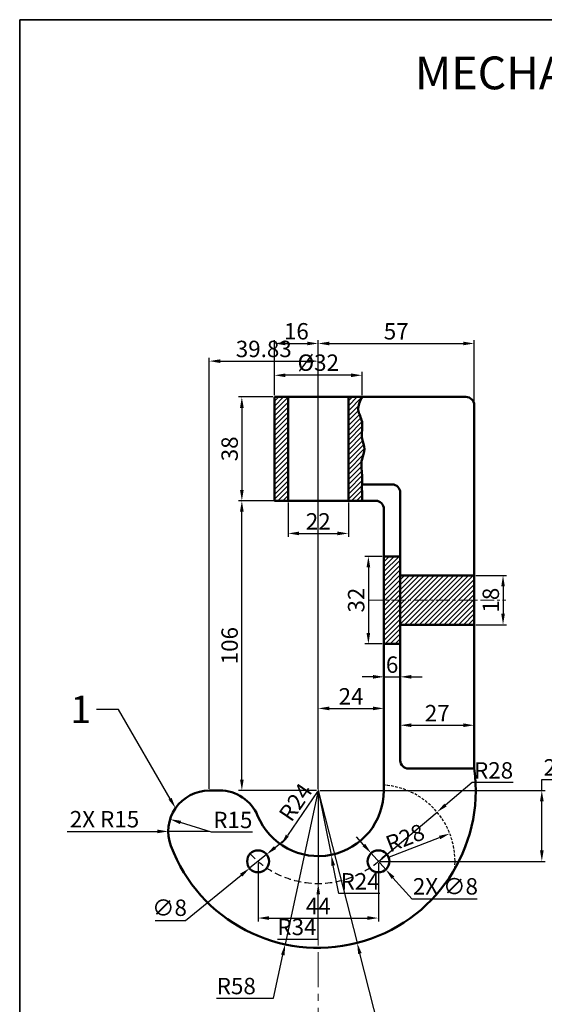
# Model space of a CAD drawing. Units: millimetres. Extents: x 44 to 571, y -292 to 291.
# Tile 2 of 4: x 44 to 236, y -69 to 291. Entities that reach past the tile are written whole.
import ezdxf
from ezdxf import colors
from ezdxf.entities.mleader import LeaderData, LeaderLine
from ezdxf.math import Vec2, Vec3

# ---------------------------------------------------------------- set-up
doc = ezdxf.new("R2010")
doc.units = ezdxf.units.MM
doc.header["$LTSCALE"] = 0.4
doc.linetypes.add('CENTER', pattern=[50.8, 31.75, -6.35, 6.35, -6.35])
doc.linetypes.add('HIDDEN', pattern=[9.525, 6.35, -3.175])
for name, color, linetype, lineweight in [('M-CNTR', 1, 'CENTER', 18), ('M-DIMS', 2, 'Continuous', 25), ('M-HATC', 8, 'Continuous', 18), ('M-HIDN', 3, 'HIDDEN', 25), ('M-OUTL', 7, 'Continuous', 50), ('M-TEXT', 3, 'Continuous', 25), ('M-TTLB', 7, 'Continuous', 35)]:
    doc.layers.add(name, color=color, linetype=linetype, lineweight=lineweight)
doc.styles.get("Standard").update_dxf_attribs({"font": 'arial.ttf'})
doc.dimstyles.new('ISO-25', dxfattribs={"dimtxt": 6, "dimasz": 4, "dimexe": 1.25, "dimexo": 0.625, "dimtad": 1, "dimtoh": 1, "dimdec": 0, "dimtxsty": 'Standard', "dimcen": 2.5, "dimadec": 0, "dimazin": 0, "dimtfac": 1, "dimtdec": 0, "dimtmove": 0, "dimatfit": 3, "dimfxl": 1, "dimarcsym": 0})

# ---------------------------------------------------------------- blocks, each defined once
blk = doc.blocks.new('*D1')
at = {"layer": 'Defpoints', "color": 0, "ltscale": 0.4, "transparency": 16777216}
for p in [(153.17, 172.64), (137.17, 153.08), (153.17, 153.08)]:
    blk.add_point(p, dxfattribs=at)
at = {"layer": 'M-DIMS', "color": 0, "lineweight": -2, "ltscale": 0.4, "transparency": 16777216}
for p, q in [((137.17, 153.7), (137.17, 173.89)), ((153.17, 153.7), (153.17, 173.89)), ((141.17, 172.64), (149.17, 172.64))]:
    blk.add_line(p, q, dxfattribs=at)
at = {"layer": 'M-DIMS', "color": 0, "ltscale": 0.4, "transparency": 16777216}
for points in [[(141.17, 173.3), (141.17, 171.97), (137.17, 172.64)], [(149.17, 173.3), (149.17, 171.97), (153.17, 172.64)]]:
    blk.add_solid(points, dxfattribs=at)
at = {"layer": 'M-DIMS', "color": 0, "ltscale": 0.4, "transparency": 16777216, "insert": (145.17, 176.32), "char_height": 6, "attachment_point": 5}
blk.add_mtext('16', dxfattribs=at)
blk = doc.blocks.new('*D2')
at = {"layer": 'Defpoints', "color": 0, "ltscale": 0.4, "transparency": 16777216}
for p in [(210.17, 172.64), (153.17, 147.48), (210.17, 143.32)]:
    blk.add_point(p, dxfattribs=at)
at = {"layer": 'M-DIMS', "color": 0, "lineweight": -2, "ltscale": 0.4, "transparency": 16777216}
for p, q in [((153.17, 148.11), (153.17, 173.89)), ((210.17, 143.94), (210.17, 173.89)), ((157.17, 172.64), (206.17, 172.64))]:
    blk.add_line(p, q, dxfattribs=at)
at = {"layer": 'M-DIMS', "color": 0, "ltscale": 0.4, "transparency": 16777216}
for points in [[(157.17, 173.3), (157.17, 171.97), (153.17, 172.64)], [(206.17, 173.3), (206.17, 171.97), (210.17, 172.64)]]:
    blk.add_solid(points, dxfattribs=at)
at = {"layer": 'M-DIMS', "color": 0, "ltscale": 0.4, "transparency": 16777216, "insert": (181.67, 176.31), "char_height": 6, "attachment_point": 5}
blk.add_mtext('57', dxfattribs=at)
blk = doc.blocks.new('*D3')
at = {"layer": 'Defpoints', "color": 0, "ltscale": 0.4, "transparency": 16777216}
for p in [(131.17, -16.85), (175.17, -16.85), (175.17, -37.59)]:
    blk.add_point(p, dxfattribs=at)
at = {"layer": 'M-DIMS', "color": 0, "lineweight": -2, "ltscale": 0.4, "transparency": 16777216}
for p, q in [((131.17, -17.47), (131.17, -38.84)), ((175.17, -17.47), (175.17, -38.84)), ((135.17, -37.59), (171.17, -37.59))]:
    blk.add_line(p, q, dxfattribs=at)
at = {"layer": 'M-DIMS', "color": 0, "ltscale": 0.4, "transparency": 16777216}
for points in [[(135.17, -36.92), (135.17, -38.26), (131.17, -37.59)], [(171.17, -36.92), (171.17, -38.26), (175.17, -37.59)]]:
    blk.add_solid(points, dxfattribs=at)
at = {"layer": 'M-DIMS', "color": 0, "ltscale": 0.4, "transparency": 16777216, "insert": (153.17, -33.97), "char_height": 6, "attachment_point": 5}
blk.add_mtext('44', dxfattribs=at)
blk = doc.blocks.new('*D4')
at = {"layer": 'Defpoints', "color": 0, "ltscale": 0.4, "transparency": 16777216}
for p in [(137.17, 153.08), (125.24, 115.08), (137.17, 115.08)]:
    blk.add_point(p, dxfattribs=at)
at = {"layer": 'M-DIMS', "color": 0, "lineweight": -2, "ltscale": 0.4, "transparency": 16777216}
for p, q in [((136.54, 153.08), (123.99, 153.08)), ((125.24, 149.08), (125.24, 119.08)), ((136.54, 115.08), (123.99, 115.08))]:
    blk.add_line(p, q, dxfattribs=at)
at = {"layer": 'M-DIMS', "color": 0, "ltscale": 0.4, "transparency": 16777216}
for points in [[(124.57, 149.08), (125.91, 149.08), (125.24, 153.08)], [(124.57, 119.08), (125.91, 119.08), (125.24, 115.08)]]:
    blk.add_solid(points, dxfattribs=at)
at = {"layer": 'M-DIMS', "color": 0, "ltscale": 0.4, "transparency": 16777216, "insert": (121.55, 134.08), "char_height": 6, "attachment_point": 5, "rotation": 90}
blk.add_mtext('38', dxfattribs=at)
blk = doc.blocks.new('*D5')
at = {"layer": 'Defpoints', "color": 0, "ltscale": 0.4, "transparency": 16777216}
for p in [(153.17, 9.08), (139.63, -10.74)]:
    blk.add_point(p, dxfattribs=at)
at = {"layer": 'M-DIMS', "color": 0, "lineweight": -2, "ltscale": 0.4, "transparency": 16777216}
blk.add_line((152.92, 8.71), (141.89, -7.44), dxfattribs=at)
at = {"layer": 'M-DIMS', "color": 0, "ltscale": 0.4, "transparency": 16777216}
blk.add_solid([(141.34, -7.07), (142.44, -7.82), (139.63, -10.74)], dxfattribs=at)
at = {"layer": 'M-DIMS', "color": 0, "ltscale": 0.4, "transparency": 16777216, "insert": (145.53, 4.34), "char_height": 6, "attachment_point": 5, "rotation": 55.6749}
blk.add_mtext('R24', dxfattribs=at)
blk = doc.blocks.new('*D6')
at = {"layer": 'Defpoints', "color": 0, "ltscale": 0.4, "transparency": 16777216}
for p in [(125.24, 115.08), (153.17, 115.08), (153.17, 9.08)]:
    blk.add_point(p, dxfattribs=at)
at = {"layer": 'M-DIMS', "color": 0, "lineweight": -2, "ltscale": 0.4, "transparency": 16777216}
for p, q in [((152.54, 115.08), (123.99, 115.08)), ((125.24, 13.08), (125.24, 111.08)), ((152.54, 9.08), (123.99, 9.08))]:
    blk.add_line(p, q, dxfattribs=at)
at = {"layer": 'M-DIMS', "color": 0, "ltscale": 0.4, "transparency": 16777216}
for points in [[(124.57, 111.08), (125.91, 111.08), (125.24, 115.08)], [(124.57, 13.08), (125.91, 13.08), (125.24, 9.08)]]:
    blk.add_solid(points, dxfattribs=at)
at = {"layer": 'M-DIMS', "color": 0, "ltscale": 0.4, "transparency": 16777216, "insert": (121.55, 62.08), "char_height": 6, "attachment_point": 5, "rotation": 90}
blk.add_mtext('106', dxfattribs=at)
blk = doc.blocks.new('*D7')
at = {"layer": 'Defpoints', "color": 0, "ltscale": 0.4, "transparency": 16777216}
for p in [(142.17, 115.08), (164.17, 115.08), (164.17, 103.14)]:
    blk.add_point(p, dxfattribs=at)
at = {"layer": 'M-DIMS', "color": 0, "lineweight": -2, "ltscale": 0.4, "transparency": 16777216}
for p, q in [((142.17, 114.45), (142.17, 101.89)), ((164.17, 114.45), (164.17, 101.89)), ((146.17, 103.14), (160.17, 103.14))]:
    blk.add_line(p, q, dxfattribs=at)
at = {"layer": 'M-DIMS', "color": 0, "ltscale": 0.4, "transparency": 16777216}
for points in [[(146.17, 103.81), (146.17, 102.47), (142.17, 103.14)], [(160.17, 103.81), (160.17, 102.47), (164.17, 103.14)]]:
    blk.add_solid(points, dxfattribs=at)
at = {"layer": 'M-DIMS', "color": 0, "ltscale": 0.4, "transparency": 16777216, "insert": (153.17, 106.78), "char_height": 6, "attachment_point": 5}
blk.add_mtext('22', dxfattribs=at)
blk = doc.blocks.new('*D8')
at = {"layer": 'Defpoints', "color": 0, "ltscale": 0.4, "transparency": 16777216}
for p in [(137.17, 161), (137.17, 153.08), (169.17, 153.08)]:
    blk.add_point(p, dxfattribs=at)
at = {"layer": 'M-DIMS', "color": 0, "lineweight": -2, "ltscale": 0.4, "transparency": 16777216}
for p, q in [((137.17, 153.7), (137.17, 162.25)), ((169.17, 153.7), (169.17, 162.25)), ((165.17, 161), (141.17, 161))]:
    blk.add_line(p, q, dxfattribs=at)
at = {"layer": 'M-DIMS', "color": 0, "ltscale": 0.4, "transparency": 16777216}
for points in [[(141.17, 161.66), (141.17, 160.33), (137.17, 161)], [(165.17, 161.66), (165.17, 160.33), (169.17, 161)]]:
    blk.add_solid(points, dxfattribs=at)
at = {"layer": 'M-DIMS', "color": 0, "ltscale": 0.4, "transparency": 16777216, "insert": (153.17, 164.85), "char_height": 6, "attachment_point": 5}
blk.add_mtext('%%C32', dxfattribs=at)
blk = doc.blocks.new('*D9')
at = {"layer": 'Defpoints', "color": 0, "ltscale": 0.4, "transparency": 16777216}
for p in [(201.26, -6.68), (175.17, -16.85)]:
    blk.add_point(p, dxfattribs=at)
at = {"layer": 'M-DIMS', "color": 0, "lineweight": -2, "ltscale": 0.4, "transparency": 16777216}
blk.add_line((179.27, -15.25), (197.53, -8.13), dxfattribs=at)
at = {"layer": 'M-DIMS', "color": 0, "ltscale": 0.4, "transparency": 16777216}
blk.add_solid([(197.29, -7.51), (197.77, -8.75), (201.26, -6.68)], dxfattribs=at)
at = {"layer": 'M-DIMS', "color": 0, "ltscale": 0.4, "transparency": 16777216, "insert": (185.2, -8.98), "char_height": 6, "attachment_point": 5, "rotation": 21.289}
blk.add_mtext('R28', dxfattribs=at)
blk = doc.blocks.new('*D10')
at = {"layer": 'Defpoints', "color": 0, "ltscale": 0.4, "transparency": 16777216}
for p in [(99.03, -1.44), (113.34, -5.92)]:
    blk.add_point(p, dxfattribs=at)
at = {"layer": 'M-DIMS', "color": 0, "lineweight": -2, "ltscale": 0.4, "transparency": 16777216}
for p, q in [((114.12, -6.17), (102.84, -2.64)), ((129.13, -6.17), (114.12, -6.17))]:
    blk.add_line(p, q, dxfattribs=at)
at = {"layer": 'M-DIMS', "color": 0, "ltscale": 0.4, "transparency": 16777216}
blk.add_solid([(103.04, -2), (102.64, -3.27), (99.03, -1.44)], dxfattribs=at)
at = {"layer": 'M-DIMS', "color": 0, "ltscale": 0.4, "transparency": 16777216, "insert": (121.94, -2.48), "char_height": 6, "attachment_point": 5}
blk.add_mtext('R15', dxfattribs=at)
blk = doc.blocks.new('*D11')
at = {"layer": 'Defpoints', "color": 0, "ltscale": 0.4, "transparency": 16777216}
for p in [(153.17, 9.08), (141.07, -47.2)]:
    blk.add_point(p, dxfattribs=at)
at = {"layer": 'M-DIMS', "color": 0, "lineweight": -2, "ltscale": 0.4, "transparency": 16777216}
for p, q in [((153.17, 9.08), (141.07, -47.2)), ((136.82, -66.94), (140.23, -51.11)), ((116.03, -66.94), (136.82, -66.94))]:
    blk.add_line(p, q, dxfattribs=at)
at = {"layer": 'M-DIMS', "color": 0, "ltscale": 0.4, "transparency": 16777216}
blk.add_solid([(139.57, -50.97), (140.88, -51.25), (141.07, -47.2)], dxfattribs=at)
at = {"layer": 'M-DIMS', "color": 0, "ltscale": 0.4, "transparency": 16777216, "insert": (123.2, -63.25), "char_height": 6, "attachment_point": 5}
blk.add_mtext('R58', dxfattribs=at)
blk = doc.blocks.new('*D12')
at = {"layer": 'Defpoints', "color": 0, "ltscale": 0.4, "transparency": 16777216}
for p in [(177.17, 39.11), (153.17, 35.46), (177.17, 35.46)]:
    blk.add_point(p, dxfattribs=at)
at = {"layer": 'M-DIMS', "color": 0, "lineweight": -2, "ltscale": 0.4, "transparency": 16777216}
for p, q in [((153.17, 36.09), (153.17, 40.36)), ((177.17, 36.09), (177.17, 40.36)), ((157.17, 39.11), (173.17, 39.11))]:
    blk.add_line(p, q, dxfattribs=at)
at = {"layer": 'M-DIMS', "color": 0, "ltscale": 0.4, "transparency": 16777216}
for points in [[(157.17, 39.78), (157.17, 38.44), (153.17, 39.11)], [(173.17, 39.78), (173.17, 38.44), (177.17, 39.11)]]:
    blk.add_solid(points, dxfattribs=at)
at = {"layer": 'M-DIMS', "color": 0, "ltscale": 0.4, "transparency": 16777216, "insert": (165.17, 42.75), "char_height": 6, "attachment_point": 5}
blk.add_mtext('24', dxfattribs=at)
blk = doc.blocks.new('*D13')
at = {"layer": 'Defpoints', "color": 0, "ltscale": 0.4, "transparency": 16777216}
for p in [(177.17, 50.67), (183.17, 50.67), (183.17, 50.67)]:
    blk.add_point(p, dxfattribs=at)
at = {"layer": 'M-DIMS', "color": 0, "lineweight": -2, "ltscale": 0.4, "transparency": 16777216}
for p, q in [((173.17, 50.67), (169.17, 50.67)), ((177.17, 51.29), (177.17, 51.92)), ((177.17, 50.67), (183.17, 50.67)), ((183.17, 51.29), (183.17, 51.92)), ((187.17, 50.67), (191.17, 50.67))]:
    blk.add_line(p, q, dxfattribs=at)
at = {"layer": 'M-DIMS', "color": 0, "ltscale": 0.4, "transparency": 16777216}
for points in [[(173.17, 51.33), (173.17, 50), (177.17, 50.67)], [(187.17, 51.33), (187.17, 50), (183.17, 50.67)]]:
    blk.add_solid(points, dxfattribs=at)
at = {"layer": 'M-DIMS', "color": 0, "ltscale": 0.4, "transparency": 16777216, "insert": (180.17, 54.36), "char_height": 6, "attachment_point": 5}
blk.add_mtext('6', dxfattribs=at)
blk = doc.blocks.new('*D14')
at = {"layer": 'Defpoints', "color": 0, "ltscale": 0.4, "transparency": 16777216}
for p in [(183.17, 32.78), (210.17, 32.96), (210.17, 32.78)]:
    blk.add_point(p, dxfattribs=at)
at = {"layer": 'M-DIMS', "color": 0, "lineweight": -2, "ltscale": 0.4, "transparency": 16777216}
for p, q in [((183.17, 33.41), (183.17, 34.21)), ((187.17, 32.96), (206.17, 32.96)), ((210.17, 33.41), (210.17, 34.21))]:
    blk.add_line(p, q, dxfattribs=at)
at = {"layer": 'M-DIMS', "color": 0, "ltscale": 0.4, "transparency": 16777216}
for points in [[(187.17, 33.63), (187.17, 32.29), (183.17, 32.96)], [(206.17, 33.63), (206.17, 32.29), (210.17, 32.96)]]:
    blk.add_solid(points, dxfattribs=at)
at = {"layer": 'M-DIMS', "color": 0, "ltscale": 0.4, "transparency": 16777216, "insert": (196.67, 36.6), "char_height": 6, "attachment_point": 5}
blk.add_mtext('27', dxfattribs=at)
blk = doc.blocks.new('*D15')
at = {"layer": 'Defpoints', "color": 0, "ltscale": 0.4, "transparency": 16777216}
for p in [(177.17, 94.73), (171.5, 62.73), (177.17, 62.73)]:
    blk.add_point(p, dxfattribs=at)
at = {"layer": 'M-DIMS', "color": 0, "lineweight": -2, "ltscale": 0.4, "transparency": 16777216}
for p, q in [((176.54, 94.73), (170.25, 94.73)), ((171.5, 90.73), (171.5, 66.73)), ((176.54, 62.73), (170.25, 62.73))]:
    blk.add_line(p, q, dxfattribs=at)
at = {"layer": 'M-DIMS', "color": 0, "ltscale": 0.4, "transparency": 16777216}
for points in [[(170.83, 90.73), (172.16, 90.73), (171.5, 94.73)], [(170.83, 66.73), (172.16, 66.73), (171.5, 62.73)]]:
    blk.add_solid(points, dxfattribs=at)
at = {"layer": 'M-DIMS', "color": 0, "ltscale": 0.4, "transparency": 16777216, "insert": (167.81, 78.73), "char_height": 6, "attachment_point": 5, "rotation": 90}
blk.add_mtext('32', dxfattribs=at)
blk = doc.blocks.new('*D16')
at = {"layer": 'Defpoints', "color": 0, "ltscale": 0.4, "transparency": 16777216}
for p in [(210.17, 87.73), (210.17, 69.73), (220.72, 69.73)]:
    blk.add_point(p, dxfattribs=at)
at = {"layer": 'M-DIMS', "color": 0, "lineweight": -2, "ltscale": 0.4, "transparency": 16777216}
for p, q in [((210.79, 87.73), (221.97, 87.73)), ((220.72, 83.73), (220.72, 73.73)), ((210.79, 69.73), (221.97, 69.73))]:
    blk.add_line(p, q, dxfattribs=at)
at = {"layer": 'M-DIMS', "color": 0, "ltscale": 0.4, "transparency": 16777216}
for points in [[(220.06, 83.73), (221.39, 83.73), (220.72, 87.73)], [(220.06, 73.73), (221.39, 73.73), (220.72, 69.73)]]:
    blk.add_solid(points, dxfattribs=at)
at = {"layer": 'M-DIMS', "color": 0, "ltscale": 0.4, "transparency": 16777216, "insert": (217.03, 78.73), "char_height": 6, "attachment_point": 5, "rotation": 90}
blk.add_mtext('18', dxfattribs=at)
blk = doc.blocks.new('*D17')
at = {"layer": 'Defpoints', "color": 0, "ltscale": 0.4, "transparency": 16777216}
for p in [(134.27, -14.32), (128.07, -19.37)]:
    blk.add_point(p, dxfattribs=at)
at = {"layer": 'M-DIMS', "color": 0, "lineweight": -2, "ltscale": 0.4, "transparency": 16777216}
for p, q in [((137.37, -11.79), (140.47, -9.27)), ((134.27, -14.32), (128.07, -19.37)), ((104.66, -38.45), (124.97, -21.9)), ((93.56, -38.45), (104.66, -38.45))]:
    blk.add_line(p, q, dxfattribs=at)
at = {"layer": 'M-DIMS', "color": 0, "ltscale": 0.4, "transparency": 16777216}
for points in [[(136.95, -11.28), (137.79, -12.31), (134.27, -14.32)], [(124.55, -21.38), (125.39, -22.42), (128.07, -19.37)]]:
    blk.add_solid(points, dxfattribs=at)
at = {"layer": 'M-DIMS', "color": 0, "ltscale": 0.4, "transparency": 16777216, "insert": (98.8, -34.59), "char_height": 6, "attachment_point": 5}
blk.add_mtext('∅8', dxfattribs=at)
blk = doc.blocks.new('*D74')
at = {"layer": 'Defpoints', "color": 0, "ltscale": 0.4, "transparency": 16777216}
for p in [(153.17, 166.18), (113.34, 9.08), (153.17, 9.08)]:
    blk.add_point(p, dxfattribs=at)
at = {"layer": 'M-DIMS', "color": 0, "lineweight": -2, "ltscale": 0.4, "transparency": 16777216}
for p, q in [((113.34, 9.7), (113.34, 167.43)), ((117.34, 166.18), (149.17, 166.18)), ((153.17, 9.7), (153.17, 167.43))]:
    blk.add_line(p, q, dxfattribs=at)
at = {"layer": 'M-DIMS', "color": 0, "ltscale": 0.4, "transparency": 16777216}
for points in [[(117.34, 166.84), (117.34, 165.51), (113.34, 166.18)], [(149.17, 166.84), (149.17, 165.51), (153.17, 166.18)]]:
    blk.add_solid(points, dxfattribs=at)
at = {"layer": 'M-DIMS', "color": 0, "ltscale": 0.4, "transparency": 16777216, "insert": (133.25, 169.87), "char_height": 6, "attachment_point": 5}
blk.add_mtext('39.83', dxfattribs=at)
blk = doc.blocks.new('*D75')
at = {"layer": 'Defpoints', "color": 0, "ltscale": 0.4, "transparency": 16777216}
for p in [(153.17, 9.08), (234.9, 9.08), (175.17, -16.85)]:
    blk.add_point(p, dxfattribs=at)
at = {"layer": 'M-DIMS', "color": 0, "lineweight": -2, "ltscale": 0.4, "transparency": 16777216}
for p, q in [((234.9, 9.08), (234.9, 13.08)), ((234.9, 13.08), (260.54, 13.08)), ((153.79, 9.08), (236.15, 9.08)), ((234.9, -12.85), (234.9, 5.08)), ((175.79, -16.85), (236.15, -16.85))]:
    blk.add_line(p, q, dxfattribs=at)
at = {"layer": 'M-DIMS', "color": 0, "ltscale": 0.4, "transparency": 16777216}
for points in [[(234.23, 5.08), (235.57, 5.08), (234.9, 9.08)], [(234.23, -12.85), (235.57, -12.85), (234.9, -16.85)]]:
    blk.add_solid(points, dxfattribs=at)
at = {"layer": 'M-DIMS', "color": 0, "ltscale": 0.4, "transparency": 16777216, "insert": (248.03, 16.77), "char_height": 6, "attachment_point": 5}
blk.add_mtext('25.923', dxfattribs=at)
blk = doc.blocks.new('*D78')
at = {"layer": 'Defpoints', "color": 0, "ltscale": 0.4, "transparency": 16777216}
for p in [(98.34, -5.9), (113.34, -5.92)]:
    blk.add_point(p, dxfattribs=at)
at = {"layer": 'M-DIMS', "color": 0, "lineweight": -2, "ltscale": 0.4, "transparency": 16777216}
for p, q in [((61.34, -5.89), (89.34, -5.89)), ((89.34, -5.89), (94.34, -5.89)), ((113.34, -5.92), (98.34, -5.9))]:
    blk.add_line(p, q, dxfattribs=at)
at = {"layer": 'M-DIMS', "color": 0, "ltscale": 0.4, "transparency": 16777216}
blk.add_solid([(94.34, -5.23), (94.34, -6.56), (98.34, -5.9)], dxfattribs=at)
at = {"layer": 'M-DIMS', "color": 0, "ltscale": 0.4, "transparency": 16777216, "insert": (75.03, -2.2), "char_height": 6, "attachment_point": 5}
blk.add_mtext('2X R15', dxfattribs=at)
blk = doc.blocks.new('*D79')
at = {"layer": 'Defpoints', "color": 0, "ltscale": 0.4, "transparency": 16777216}
for p in [(153.17, 9.08), (157.87, -14.46)]:
    blk.add_point(p, dxfattribs=at)
at = {"layer": 'M-DIMS', "color": 0, "lineweight": -2, "ltscale": 0.4, "transparency": 16777216}
for p, q in [((153.17, 9.08), (157.87, -14.46)), ((160.7, -28.58), (158.66, -18.38)), ((175.64, -28.58), (160.7, -28.58))]:
    blk.add_line(p, q, dxfattribs=at)
at = {"layer": 'M-DIMS', "color": 0, "ltscale": 0.4, "transparency": 16777216}
blk.add_solid([(159.31, -18.25), (158.01, -18.51), (157.87, -14.46)], dxfattribs=at)
at = {"layer": 'M-DIMS', "color": 0, "ltscale": 0.4, "transparency": 16777216, "insert": (168.48, -24.94), "char_height": 6, "attachment_point": 5}
blk.add_mtext('R24', dxfattribs=at)
blk = doc.blocks.new('*D80')
at = {"layer": 'Defpoints', "color": 0, "ltscale": 0.4, "transparency": 16777216}
for p in [(196.6, 1.17), (175.17, -16.85)]:
    blk.add_point(p, dxfattribs=at)
at = {"layer": 'M-DIMS', "color": 0, "lineweight": -2, "ltscale": 0.4, "transparency": 16777216}
for p, q in [((209.47, 11.97), (199.67, 3.74)), ((224.44, 11.97), (209.47, 11.97)), ((175.17, -16.85), (196.6, 1.17))]:
    blk.add_line(p, q, dxfattribs=at)
at = {"layer": 'M-DIMS', "color": 0, "ltscale": 0.4, "transparency": 16777216}
blk.add_solid([(199.24, 4.25), (200.1, 3.23), (196.6, 1.17)], dxfattribs=at)
at = {"layer": 'M-DIMS', "color": 0, "ltscale": 0.4, "transparency": 16777216, "insert": (217.27, 15.66), "char_height": 6, "attachment_point": 5}
blk.add_mtext('R28', dxfattribs=at)
blk = doc.blocks.new('*D81')
at = {"layer": 'Defpoints', "color": 0, "ltscale": 0.4, "transparency": 16777216}
for p in [(153.17, 9.08), (167.4, -46.7)]:
    blk.add_point(p, dxfattribs=at)
at = {"layer": 'M-DIMS', "color": 0, "lineweight": -2, "ltscale": 0.4, "transparency": 16777216}
for p, q in [((153.17, 9.08), (167.4, -46.7)), ((175.94, -80.16), (168.39, -50.57)), ((202.55, -80.16), (175.94, -80.16))]:
    blk.add_line(p, q, dxfattribs=at)
at = {"layer": 'M-DIMS', "color": 0, "ltscale": 0.4, "transparency": 16777216}
blk.add_solid([(169.03, -50.41), (167.74, -50.74), (167.4, -46.7)], dxfattribs=at)
at = {"layer": 'M-DIMS', "color": 0, "ltscale": 0.4, "transparency": 16777216, "insert": (189.55, -76.47), "char_height": 6, "attachment_point": 5}
blk.add_mtext('R57.56', dxfattribs=at)
blk = doc.blocks.new('*D82')
at = {"layer": 'Defpoints', "color": 0, "ltscale": 0.4, "transparency": 16777216}
for p in [(153.17, 9.08), (153.17, -24.92)]:
    blk.add_point(p, dxfattribs=at)
at = {"layer": 'M-DIMS', "color": 0, "lineweight": -2, "ltscale": 0.4, "transparency": 16777216}
for p, q in [((153.17, 9.08), (153.17, -24.92)), ((153.17, -45.32), (153.17, -28.92)), ((138.23, -45.32), (153.17, -45.32))]:
    blk.add_line(p, q, dxfattribs=at)
at = {"layer": 'M-DIMS', "color": 0, "ltscale": 0.4, "transparency": 16777216}
blk.add_solid([(152.5, -28.92), (153.83, -28.92), (153.17, -24.92)], dxfattribs=at)
at = {"layer": 'M-DIMS', "color": 0, "ltscale": 0.4, "transparency": 16777216, "insert": (145.39, -41.63), "char_height": 6, "attachment_point": 5}
blk.add_mtext('R34', dxfattribs=at)
blk = doc.blocks.new('*D83')
at = {"layer": 'Defpoints', "color": 0, "ltscale": 0.4, "transparency": 16777216}
for p in [(172.51, -13.86), (177.83, -19.83)]:
    blk.add_point(p, dxfattribs=at)
at = {"layer": 'M-DIMS', "color": 0, "lineweight": -2, "ltscale": 0.4, "transparency": 16777216}
for p, q in [((169.85, -10.87), (167.18, -7.89)), ((172.51, -13.86), (177.83, -19.83)), ((187.45, -30.63), (180.49, -22.82)), ((211.23, -30.63), (187.45, -30.63))]:
    blk.add_line(p, q, dxfattribs=at)
at = {"layer": 'M-DIMS', "color": 0, "ltscale": 0.4, "transparency": 16777216}
for points in [[(170.34, -10.43), (169.35, -11.32), (172.51, -13.86)], [(180.99, -22.38), (179.99, -23.26), (177.83, -19.83)]]:
    blk.add_solid(points, dxfattribs=at)
at = {"layer": 'M-DIMS', "color": 0, "ltscale": 0.4, "transparency": 16777216, "insert": (199.65, -26.77), "char_height": 6, "attachment_point": 5}
blk.add_mtext('2X ∅8', dxfattribs=at)

msp = doc.modelspace()

# ---------------------------------------------------------------- hatches: boundary and pattern name
at = {"layer": 'M-HATC', "ltscale": 0.4}
h = msp.add_hatch(dxfattribs=at)
h.set_pattern_fill('ANSI31', color=256, scale=0.4)
h.paths.add_polyline_path([(466.6963, 51.668), (466.6963, 51.668, 0.41365763), (455.6963, 51.668, 0.41365763)])
h.paths.add_polyline_path([(444.6963, 91.3959, 0.41365763), (455.6963, 91.3959, 0.41365763)])
h.paths.add_polyline_path([(171.2864, 238.6681), (441.8676, 238.6681), (441.8676, 283.6094), (171.2864, 283.6094)], flags=9)
h = msp.add_hatch(dxfattribs=at)
h.set_pattern_fill('ANSI31', color=256, scale=0.4)
h.paths.add_polyline_path([(142.1682, 153.0761), (137.1682, 153.0761), (137.1682, 115.0761), (142.1682, 115.0761)])
edge = h.paths.add_edge_path()
edge.add_spline(control_points=[(169.1682, 121.0761), (169.1831, 122.2349), (169.2918, 125.3014), (168.4842, 129.7015), (170.7826, 134.0186), (168.3045, 138.4778), (170.1262, 143.5417), (166.9696, 148.4441), (168.42, 151.4999), (169.1682, 153.0761)], knot_values=[0, 0, 0, 0, 3.48000524, 9.22344654, 13.02049624, 16.94335073, 23.13672166, 27.73131439, 32.62610012, 32.62610012, 32.62610012, 32.62610012], degree=3, periodic=0)
edge.add_line((169.1682, 153.0761), (164.1682, 153.0761))
edge.add_line((164.1682, 153.0761), (164.1682, 115.0761))
edge.add_line((164.1682, 115.0761), (169.1682, 115.0761))
edge.add_spline(control_points=[(169.1682, 115.0761), (169.1695, 115.9082), (169.1726, 117.908), (169.1532, 119.9094), (169.1682, 121.0761)], knot_values=[32.62610012, 32.62610012, 32.62610012, 32.62610012, 35.12278801, 38.62610012, 38.62610012, 38.62610012, 38.62610012], degree=3, periodic=0)
h = msp.add_hatch(dxfattribs=at)
h.set_pattern_fill('ANSI31', color=256, scale=0.4)
h.paths.add_polyline_path([(210.1682, 87.7257), (183.1682, 87.7257), (183.1682, 78.7257), (210.1682, 78.7257)])
h.paths.add_polyline_path([(210.1682, 78.7257), (183.1682, 78.7257), (183.1682, 69.7257), (210.1682, 69.7257)])
h.paths.add_polyline_path([(183.1682, 87.7257), (183.1682, 94.7257), (177.1682, 94.7257), (177.1682, 78.7257), (183.1682, 78.7257)])
h.paths.add_polyline_path([(183.1682, 78.7257), (177.1682, 78.7257), (177.1682, 62.7257), (183.1682, 62.7257)])

# ---------------------------------------------------------------- linework, layer by layer
at = {"layer": 'M-CNTR'}
msp.add_line((153.1682, 153.0761), (153.1682, -73.3053), dxfattribs=at)
at = {"layer": 'M-CNTR', "ltscale": 0.4}
msp.add_line((171.806, 78.7257), (221.7992, 78.7257), dxfattribs=at)
at = {"layer": 'M-HIDN', "ltscale": 0.4}
msp.add_arc((175.1682, -16.8469), 28, 354.17373, 85.903956, dxfattribs=at)
at = {"layer": 'M-HIDN'}
msp.add_arc((153.1682, 9.0761), 34, 222.935212, 317.064788, dxfattribs=at)
at = {"layer": 'M-OUTL'}
for p, q in [((137.1682, 153.0761), (207.1682, 153.0761)), ((137.1682, 153.0761), (137.1682, 115.0761)), ((169.1682, 121.0761), (180.1682, 121.0761)), ((183.1682, 118.0761), (183.1682, 20.0761)), ((137.1682, 115.0761), (174.1682, 115.0761)), ((177.1682, 112.0761), (177.1682, 9.0761)), ((117.1682, 9.0761), (113.3406, 9.0761))]:
    msp.add_line(p, q, dxfattribs=at)
at = {"layer": 'M-OUTL', "ltscale": 0.4}
for p, q in [((142.1682, 153.0761), (142.1682, 115.0761)), ((164.1682, 153.0761), (164.1682, 115.0761)), ((210.1682, 150.0761), (210.1682, 17.0761)), ((177.1682, 94.7257), (183.1682, 94.7257)), ((183.1682, 87.7257), (210.1682, 87.7257)), ((183.1682, 69.7257), (210.1682, 69.7257)), ((177.1682, 62.7257), (183.1682, 62.7257)), ((210.1682, 17.0761), (186.1682, 17.0761))]:
    msp.add_line(p, q, dxfattribs=at)
at = {"layer": 'M-OUTL'}
for centre in [(131.1682, -16.8469), (175.1682, -16.8469)]:
    msp.add_circle(centre, 4, dxfattribs=at)
at = {"layer": 'M-OUTL', "ltscale": 0.4}
for centre, radius, start, end in [((207.1682, 150.0761), 3, 0, 90), ((186.1682, 20.0761), 3, 180, 270), ((153.1682, 9.0761), 57.5587, 200.637527, 7.989327), ((113.3406, -5.9239), 15, 90, 200.637527)]:
    msp.add_arc(centre, radius, start, end, dxfattribs=at)
at = {"layer": 'M-OUTL'}
for centre, radius, start, end in [((180.1682, 118.0761), 3, 0, 90), ((174.1682, 112.0761), 3, 0, 90), ((117.1682, -5.9239), 15, 22.619865, 90), ((153.1682, 9.0761), 24, 202.619865, 0)]:
    msp.add_arc(centre, radius, start, end, dxfattribs=at)
at = {"layer": 'M-OUTL', "ltscale": 0.4}
msp.add_open_spline([(169.1682, 153.0761), (168.42, 151.4999), (166.9696, 148.4441), (170.1262, 143.5417), (168.3045, 138.4778), (170.7826, 134.0186), (168.4842, 129.7015), (169.2918, 125.3014), (169.1419, 121.0702), (169.1726, 117.908), (169.1695, 115.9082), (169.1682, 115.0761)], degree=3, knots=[0, 0, 0, 0, 4.89478572, 9.48937846, 15.68274938, 19.60560388, 23.40265357, 29.14609488, 32.62610012, 36.12941222, 38.62610012, 38.62610012, 38.62610012, 38.62610012], dxfattribs=at)
at = {"layer": 'M-TTLB', "ltscale": 0.4}
msp.add_lwpolyline([(44.037, 291.1069), (570.566, 291.1069), (570.566, -292.0762), (44.037, -292.0762)], close=True, dxfattribs=at)

# ---------------------------------------------------------------- texts
at = {"layer": 'M-TTLB', "ltscale": 0.4, "insert": (142.2261, 277.638), "char_height": 12, "attachment_point": 1}
msp.add_mtext_dynamic_manual_height_columns('\\pxqc;MECHANICAL LEVER ASSEMBLY COMPONENTS', width=329.81502, gutter_width=12.5, heights=[0], dxfattribs=at)

# ---------------------------------------------------------------- dimensions: what is measured, and where the dimension line sits
at = {"layer": 'M-DIMS', "ltscale": 0.4}
dim = msp.add_linear_dim(base=(153.1682, 172.6358), p1=(137.1682, 153.0761), p2=(153.1682, 153.0761), dimstyle='ISO-25', override={"dimclrd": 0, "dimclre": 0, "dimclrt": 0}, dxfattribs=at)
dim.commit()
dim.dimension.update_dxf_attribs({"geometry": '*D1', "text_midpoint": (145.1682, 172.6358), "dimtype": 160})
for base, p1, p2, override, picture, middle in [((210.1682, 172.6358), (153.1682, 147.4801), (210.1682, 143.3191), {"dimclrd": 0, "dimclre": 0, "dimclrt": 0}, '*D2', (181.6682, 176.312)), ((153.1682, 166.1761), (113.3406, 9.0761), (153.1682, 9.0761), {"dimdec": 2, "dimlfac": 1, "dimrnd": 0, "dimzin": 0, "dimdsep": 46, "dimlunit": 2}, '*D74', (133.2544, 169.8665)), ((164.1682, 103.1404), (142.1682, 115.0761), (164.1682, 115.0761), {"dimclrd": 0, "dimclre": 0, "dimclrt": 0}, '*D7', (153.1682, 106.7777)), ((183.1682, 50.667), (177.1682, 50.667), (183.1682, 50.667), {"dimclrd": 0, "dimclre": 0, "dimclrt": 0}, '*D13', (180.1682, 54.3555)), ((177.1682, 39.109), (153.1682, 35.4634), (177.1682, 35.4634), {"dimclrd": 0, "dimclre": 0, "dimclrt": 0}, '*D12', (165.1682, 42.7463)), ((210.1682, 32.9616), (183.1682, 32.7823), (210.1682, 32.7823), {"dimclrd": 0, "dimclre": 0, "dimclrt": 0}, '*D14', (196.6682, 36.5989)), ((175.1682, -37.5911), (131.1682, -16.8469), (175.1682, -16.8469), {"dimclrd": 0, "dimclre": 0, "dimclrt": 0}, '*D3', (153.1682, -33.9661))]:
    dim = msp.add_linear_dim(base=base, p1=p1, p2=p2, dimstyle='ISO-25', override=override, dxfattribs=at)
    dim.commit()
    dim.dimension.update_dxf_attribs({"geometry": picture, "text_midpoint": middle})
dim = msp.add_linear_dim(base=(137.1682, 160.9955), p1=(169.1682, 153.0761), p2=(137.1682, 153.0761), text='%%C<>', dimstyle='ISO-25', override={"dimclrd": 0, "dimclre": 0, "dimclrt": 0}, dxfattribs=at)
dim.commit()
dim.dimension.update_dxf_attribs({"geometry": '*D8', "text_midpoint": (153.1682, 160.9955), "dimtype": 160})
for base, p1, p2, override, picture, middle in [((125.2405, 115.0761), (137.1682, 153.0761), (137.1682, 115.0761), {"dimclrd": 0, "dimclre": 0, "dimclrt": 0}, '*D4', (121.55, 134.0761)), ((125.2405, 115.0761), (153.1682, 9.0761), (153.1682, 115.0761), {"dimclrd": 0, "dimclre": 0, "dimclrt": 0}, '*D6', (121.5521, 62.0761)), ((171.4968, 62.7257), (177.1682, 94.7257), (177.1682, 62.7257), {"dimclrd": 0, "dimclre": 0, "dimclrt": 0}, '*D15', (167.8063, 78.7257)), ((220.7218, 69.7257), (210.1682, 87.7257), (210.1682, 69.7257), {"dimclrd": 0, "dimclre": 0, "dimclrt": 0}, '*D16', (217.0333, 78.7257)), ((234.8992, 9.0761), (175.1682, -16.8469), (153.1682, 9.0761), {"dimdec": 3, "dimlfac": 1, "dimrnd": 0, "dimzin": 0, "dimdsep": 46, "dimlunit": 2}, '*D75', (248.0297, 16.7665))]:
    dim = msp.add_linear_dim(base=base, p1=p1, p2=p2, angle=90, dimstyle='ISO-25', override=override, dxfattribs=at)
    dim.commit()
    dim.dimension.update_dxf_attribs({"geometry": picture, "text_midpoint": middle})
for center, mpoint, override, picture, middle in [((175.1682, -16.8469), (196.605, 1.166), {"dimdec": 0, "dimlfac": 1, "dimrnd": 0, "dimzin": 0, "dimdsep": 46, "dimlunit": 2}, '*D80', (217.2667, 11.9737)), ((153.1682, 9.0761), (139.6349, -10.7444), {"dimclrd": 0, "dimclre": 0, "dimclrt": 0}, '*D5', (148.5337, 2.2886)), ((153.1682, 9.0761), (141.0674, -47.1962), {"dimclrd": 0, "dimclre": 0, "dimclrt": 0}, '*D11', (123.2045, -66.9386)), ((153.1682, 9.0761), (153.168, -24.9239), {"dimdec": 0, "dimlfac": 1, "dimrnd": 0, "dimzin": 0, "dimdsep": 46, "dimlunit": 2}, '*D82', (145.3867, -45.3239)), ((153.1682, 9.0761), (157.875, -14.4579), {"dimdec": 0, "dimlfac": 1, "dimrnd": 0, "dimzin": 0, "dimdsep": 46, "dimlunit": 2}, '*D79', (168.4802, -28.5782)), ((153.1682, 9.0761), (167.398, -46.6959), {"dimdec": 2, "dimlfac": 1, "dimrnd": 0, "dimzin": 0, "dimdsep": 46, "dimlunit": 2}, '*D81', (189.5533, -80.1591)), ((113.3406, -5.9239), (99.0259, -1.4418), {"dimclrd": 0, "dimclre": 0, "dimclrt": 0}, '*D10', (121.9353, -6.1678)), ((175.1682, -16.8469), (201.2575, -6.6809), {"dimclrd": 0, "dimclre": 0, "dimclrt": 0}, '*D9', (186.536, -12.4173))]:
    dim = msp.add_radius_dim(center=center, mpoint=mpoint, dimstyle='ISO-25', override=override, dxfattribs=at)
    dim.commit()
    dim.dimension.update_dxf_attribs({"geometry": picture, "text_midpoint": middle, "dimtype": 164})
dim = msp.add_radius_dim(center=(113.3406, -5.9239), mpoint=(98.3406, -5.8997), text='2X <>', dimstyle='ISO-25', override={"dimdec": 0, "dimlfac": 1, "dimrnd": 0, "dimzin": 0, "dimdsep": 46, "dimlunit": 2}, dxfattribs=at)
dim.commit()
dim.dimension.update_dxf_attribs({"geometry": '*D78', "text_midpoint": (89.3406, -5.8852), "dimtype": 164})
dim = msp.add_diameter_dim_2p(p1=(134.2689, -14.3199), p2=(128.0675, -19.3739), dimstyle='ISO-25', override={"dimclrd": 0, "dimclre": 0, "dimclrt": 0}, dxfattribs=at)
dim.commit()
dim.dimension.update_dxf_attribs({"geometry": '*D17', "text_midpoint": (98.8, -38.4496), "dimtype": 163})
dim = msp.add_diameter_dim_2p(p1=(172.5069, -13.8607), p2=(177.8295, -19.8331), text='2X <>', dimstyle='ISO-25', override={"dimdec": 0, "dimlfac": 1, "dimrnd": 0, "dimzin": 0, "dimdsep": 46, "dimlunit": 2}, dxfattribs=at)
dim.commit()
dim.dimension.update_dxf_attribs({"geometry": '*D83', "text_midpoint": (199.6511, -30.6301), "dimtype": 163})

# ---------------------------------------------------------------- leaders
at = {"layer": 'M-TEXT', "ltscale": 0.4}
ml = msp.add_multileader_mtext('Standard', dxfattribs=at)
ml.set_content('1', color=256)
ml.set_leader_properties()
ml.build(insert=Vec2(0, 0))
ctx = ml.context
ctx.base_point, ctx.char_height, ctx.plane_origin = Vec3(64.4527, 38.7582), 10, Vec3(101.0056, 2.6112)
ctx.text_align_type = 2
notes = []
notes.append((ctx, [(0, (1, 1, 0), (80.1362, 38.7582), (-1, 0), 8, [(0, [(101.0056, 2.6112)], 0, [])])]))
ctx.mtext.insert, ctx.mtext.alignment, ctx.mtext.flow_direction = Vec3(70.1362, 43.7582), 3, 5
for ctx, leaders in notes:
    for number, flags, end, landing, length, lines in leaders:
        leader = LeaderData()
        leader.index, (leader.has_last_leader_line, leader.has_dogleg_vector, leader.attachment_direction) = number, flags
        leader.last_leader_point, leader.dogleg_vector, leader.dogleg_length = Vec3(end), Vec3(landing), length
        for number, points, colour, breaks in lines:
            line = LeaderLine()
            line.index, line.vertices, line.color, line.breaks = number, Vec3.list(points), colors.encode_raw_color(colour), breaks
            leader.lines.append(line)
        ctx.leaders.append(leader)

doc.saveas('drawing.dxf')
